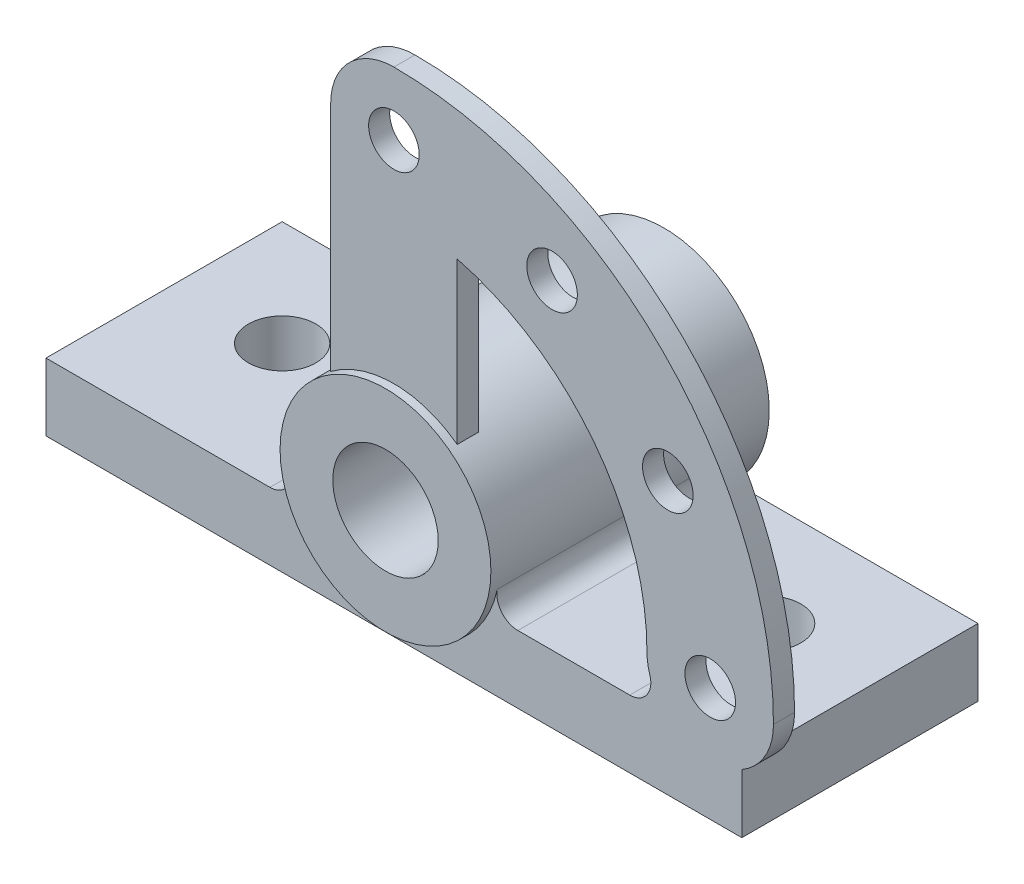
ISO-10303-21;
HEADER;
FILE_DESCRIPTION(('STEP AP214'),'2;1');
FILE_NAME('part.step','',(''),(''),'','','');
FILE_SCHEMA(('AUTOMOTIVE_DESIGN { 1 0 10303 214 1 1 1 1 }'));
ENDSEC;
DATA;
#1=APPLICATION_CONTEXT('core data for automotive mechanical design processes');
#2=APPLICATION_PROTOCOL_DEFINITION('international standard','automotive_design',2000,#1);
#3=PRODUCT_CONTEXT('',#1,'mechanical');
#4=PRODUCT('Part','Part','',(#3));
#5=PRODUCT_RELATED_PRODUCT_CATEGORY('part','',(#4));
#6=PRODUCT_DEFINITION_FORMATION('','',#4);
#7=PRODUCT_DEFINITION_CONTEXT('part definition',#1,'design');
#8=PRODUCT_DEFINITION('design','',#6,#7);
#9=PRODUCT_DEFINITION_SHAPE('','',#8);
#10=(LENGTH_UNIT() NAMED_UNIT(*) SI_UNIT(.MILLI.,.METRE.));
#11=(NAMED_UNIT(*) PLANE_ANGLE_UNIT() SI_UNIT($,.RADIAN.));
#12=(NAMED_UNIT(*) SI_UNIT($,.STERADIAN.) SOLID_ANGLE_UNIT());
#13=UNCERTAINTY_MEASURE_WITH_UNIT(LENGTH_MEASURE(1.E-05),#10,'distance_accuracy_value','');
#14=(GEOMETRIC_REPRESENTATION_CONTEXT(3) GLOBAL_UNCERTAINTY_ASSIGNED_CONTEXT((#13)) GLOBAL_UNIT_ASSIGNED_CONTEXT((#10,
#11,#12)) REPRESENTATION_CONTEXT('',''));
#15=CARTESIAN_POINT('',(0.,0.,0.));
#16=DIRECTION('',(0.,0.,1.));
#17=DIRECTION('',(1.,0.,0.));
#18=AXIS2_PLACEMENT_3D('',#15,#16,#17);
#19=CARTESIAN_POINT('',(165.,16.,56.));
#20=DIRECTION('',(0.,-1.,0.));
#21=DIRECTION('',(0.,0.,-1.));
#22=AXIS2_PLACEMENT_3D('',#19,#20,#21);
#23=PLANE('',#22);
#24=CARTESIAN_POINT('',(140.,16.,25.));
#25=DIRECTION('',(0.,1.,0.));
#26=DIRECTION('',(0.,0.,1.));
#27=AXIS2_PLACEMENT_3D('',#24,#25,#26);
#28=CIRCLE('',#27,8.00000000000001);
#29=CARTESIAN_POINT('',(140.,16.,33.));
#30=VERTEX_POINT('',#29);
#31=EDGE_CURVE('E445',#30,#30,#28,.T.);
#32=ORIENTED_EDGE('',*,*,#31,.F.);
#33=EDGE_LOOP('',(#32));
#34=FACE_BOUND('',#33,.T.);
#35=DIRECTION('',(-1.,0.,0.));
#36=VECTOR('',#35,1.);
#37=CARTESIAN_POINT('',(165.,16.,56.));
#38=LINE('',#37,#36);
#39=CARTESIAN_POINT('',(138.421215971661,16.,56.));
#40=VERTEX_POINT('',#39);
#41=CARTESIAN_POINT('',(111.893876913398,16.,56.));
#42=VERTEX_POINT('',#41);
#43=EDGE_CURVE('E291',#40,#42,#38,.T.);
#44=ORIENTED_EDGE('',*,*,#43,.F.);
#45=DIRECTION('',(0.,0.,1.));
#46=VECTOR('',#45,1.);
#47=CARTESIAN_POINT('',(138.421215971661,16.,51.));
#48=LINE('',#47,#46);
#49=CARTESIAN_POINT('',(138.421215971661,16.,51.));
#50=VERTEX_POINT('',#49);
#51=EDGE_CURVE('E333',#40,#50,#48,.F.);
#52=ORIENTED_EDGE('',*,*,#51,.T.);
#53=DIRECTION('',(-1.,0.,0.));
#54=VECTOR('',#53,1.);
#55=CARTESIAN_POINT('',(165.,16.,51.));
#56=LINE('',#55,#54);
#57=CARTESIAN_POINT('',(165.,16.,51.));
#58=VERTEX_POINT('',#57);
#59=EDGE_CURVE('E264',#58,#50,#56,.T.);
#60=ORIENTED_EDGE('',*,*,#59,.F.);
#61=DIRECTION('',(0.,0.,-1.));
#62=VECTOR('',#61,1.);
#63=CARTESIAN_POINT('',(165.,16.,56.));
#64=LINE('',#63,#62);
#65=CARTESIAN_POINT('',(165.,16.,0.));
#66=VERTEX_POINT('',#65);
#67=EDGE_CURVE('E307',#58,#66,#64,.T.);
#68=ORIENTED_EDGE('',*,*,#67,.T.);
#69=DIRECTION('',(-1.,0.,0.));
#70=VECTOR('',#69,1.);
#71=CARTESIAN_POINT('',(165.,16.,0.));
#72=LINE('',#71,#70);
#73=CARTESIAN_POINT('',(111.893876913398,16.,0.));
#74=VERTEX_POINT('',#73);
#75=EDGE_CURVE('E290',#66,#74,#72,.T.);
#76=ORIENTED_EDGE('',*,*,#75,.T.);
#77=DIRECTION('',(0.,0.,1.));
#78=VECTOR('',#77,1.);
#79=CARTESIAN_POINT('',(111.893876913398,16.,56.));
#80=LINE('',#79,#78);
#81=EDGE_CURVE('E329',#74,#42,#80,.T.);
#82=ORIENTED_EDGE('',*,*,#81,.T.);
#83=EDGE_LOOP('',(#44,#52,#60,#68,#76,#82));
#84=FACE_BOUND('',#83,.T.);
#85=ADVANCED_FACE('F43',(#34,#84),#23,.F.);
#86=CARTESIAN_POINT('',(165.,0.,56.));
#87=DIRECTION('',(-1.,0.,0.));
#88=DIRECTION('',(0.,0.,1.));
#89=AXIS2_PLACEMENT_3D('',#86,#87,#88);
#90=PLANE('',#89);
#91=DIRECTION('',(0.,0.,-1.));
#92=VECTOR('',#91,1.);
#93=CARTESIAN_POINT('',(165.,14.0096189432334,56.));
#94=LINE('',#93,#92);
#95=CARTESIAN_POINT('',(165.,14.0096189432334,56.));
#96=VERTEX_POINT('',#95);
#97=CARTESIAN_POINT('',(165.,14.0096189432334,51.));
#98=VERTEX_POINT('',#97);
#99=EDGE_CURVE('E268',#96,#98,#94,.T.);
#100=ORIENTED_EDGE('',*,*,#99,.F.);
#101=DIRECTION('',(0.,1.,0.));
#102=VECTOR('',#101,1.);
#103=CARTESIAN_POINT('',(165.,0.,56.));
#104=LINE('',#103,#102);
#105=CARTESIAN_POINT('',(165.,0.,56.));
#106=VERTEX_POINT('',#105);
#107=EDGE_CURVE('E287',#106,#96,#104,.T.);
#108=ORIENTED_EDGE('',*,*,#107,.F.);
#109=DIRECTION('',(0.,0.,-1.));
#110=VECTOR('',#109,1.);
#111=CARTESIAN_POINT('',(165.,0.,56.));
#112=LINE('',#111,#110);
#113=CARTESIAN_POINT('',(165.,0.,0.));
#114=VERTEX_POINT('',#113);
#115=EDGE_CURVE('E311',#106,#114,#112,.T.);
#116=ORIENTED_EDGE('',*,*,#115,.T.);
#117=DIRECTION('',(0.,1.,0.));
#118=VECTOR('',#117,1.);
#119=CARTESIAN_POINT('',(165.,0.,0.));
#120=LINE('',#119,#118);
#121=EDGE_CURVE('E301',#114,#66,#120,.T.);
#122=ORIENTED_EDGE('',*,*,#121,.T.);
#123=ORIENTED_EDGE('',*,*,#67,.F.);
#124=DIRECTION('',(0.,1.,0.));
#125=VECTOR('',#124,1.);
#126=CARTESIAN_POINT('',(165.,0.,51.));
#127=LINE('',#126,#125);
#128=EDGE_CURVE('E263',#98,#58,#127,.T.);
#129=ORIENTED_EDGE('',*,*,#128,.F.);
#130=EDGE_LOOP('',(#100,#108,#116,#122,#123,#129));
#131=FACE_BOUND('',#130,.T.);
#132=ADVANCED_FACE('F380',(#131),#90,.F.);
#133=CARTESIAN_POINT('',(25.,16.,25.));
#134=DIRECTION('',(0.,1.,0.));
#135=DIRECTION('',(0.,0.,1.));
#136=AXIS2_PLACEMENT_3D('',#133,#134,#135);
#137=CIRCLE('',#136,8.);
#138=CARTESIAN_POINT('',(25.,16.,33.));
#139=VERTEX_POINT('',#138);
#140=EDGE_CURVE('E401',#139,#139,#137,.T.);
#141=ORIENTED_EDGE('',*,*,#140,.F.);
#142=EDGE_LOOP('',(#141));
#143=FACE_BOUND('',#142,.T.);
#144=CARTESIAN_POINT('',(53.1061230866019,16.,56.));
#145=VERTEX_POINT('',#144);
#146=CARTESIAN_POINT('',(0.,16.,56.));
#147=VERTEX_POINT('',#146);
#148=EDGE_CURVE('E292',#145,#147,#38,.T.);
#149=ORIENTED_EDGE('',*,*,#148,.F.);
#150=DIRECTION('',(0.,0.,1.));
#151=VECTOR('',#150,1.);
#152=CARTESIAN_POINT('',(53.1061230866019,16.,0.));
#153=LINE('',#152,#151);
#154=CARTESIAN_POINT('',(53.1061230866019,16.,0.));
#155=VERTEX_POINT('',#154);
#156=EDGE_CURVE('E318',#145,#155,#153,.F.);
#157=ORIENTED_EDGE('',*,*,#156,.T.);
#158=CARTESIAN_POINT('',(0.,16.,0.));
#159=VERTEX_POINT('',#158);
#160=EDGE_CURVE('E302',#155,#159,#72,.T.);
#161=ORIENTED_EDGE('',*,*,#160,.T.);
#162=DIRECTION('',(0.,0.,-1.));
#163=VECTOR('',#162,1.);
#164=CARTESIAN_POINT('',(0.,16.,56.));
#165=LINE('',#164,#163);
#166=EDGE_CURVE('E298',#147,#159,#165,.T.);
#167=ORIENTED_EDGE('',*,*,#166,.F.);
#168=EDGE_LOOP('',(#149,#157,#161,#167));
#169=FACE_BOUND('',#168,.T.);
#170=ADVANCED_FACE('F379',(#143,#169),#23,.F.);
#171=CARTESIAN_POINT('',(0.,16.,56.));
#172=DIRECTION('',(1.,0.,0.));
#173=DIRECTION('',(0.,0.,-1.));
#174=AXIS2_PLACEMENT_3D('',#171,#172,#173);
#175=PLANE('',#174);
#176=DIRECTION('',(0.,-1.,0.));
#177=VECTOR('',#176,1.);
#178=CARTESIAN_POINT('',(0.,16.,0.));
#179=LINE('',#178,#177);
#180=CARTESIAN_POINT('',(0.,0.,0.));
#181=VERTEX_POINT('',#180);
#182=EDGE_CURVE('E285',#159,#181,#179,.T.);
#183=ORIENTED_EDGE('',*,*,#182,.T.);
#184=DIRECTION('',(0.,0.,-1.));
#185=VECTOR('',#184,1.);
#186=CARTESIAN_POINT('',(0.,0.,56.));
#187=LINE('',#186,#185);
#188=CARTESIAN_POINT('',(0.,0.,56.));
#189=VERTEX_POINT('',#188);
#190=EDGE_CURVE('E313',#189,#181,#187,.T.);
#191=ORIENTED_EDGE('',*,*,#190,.F.);
#192=DIRECTION('',(0.,-1.,0.));
#193=VECTOR('',#192,1.);
#194=CARTESIAN_POINT('',(0.,16.,56.));
#195=LINE('',#194,#193);
#196=EDGE_CURVE('E281',#147,#189,#195,.T.);
#197=ORIENTED_EDGE('',*,*,#196,.F.);
#198=ORIENTED_EDGE('',*,*,#166,.T.);
#199=EDGE_LOOP('',(#183,#191,#197,#198));
#200=FACE_BOUND('',#199,.T.);
#201=ADVANCED_FACE('F393',(#200),#175,.F.);
#202=CARTESIAN_POINT('',(75.,0.,56.));
#203=DIRECTION('',(0.,1.,0.));
#204=DIRECTION('',(0.,0.,1.));
#205=AXIS2_PLACEMENT_3D('',#202,#203,#204);
#206=PLANE('',#205);
#207=CARTESIAN_POINT('',(140.,0.,25.));
#208=DIRECTION('',(0.,1.,0.));
#209=DIRECTION('',(0.,0.,1.));
#210=AXIS2_PLACEMENT_3D('',#207,#208,#209);
#211=CIRCLE('',#210,8.00000000000001);
#212=CARTESIAN_POINT('',(140.,0.,33.));
#213=VERTEX_POINT('',#212);
#214=EDGE_CURVE('E437',#213,#213,#211,.T.);
#215=ORIENTED_EDGE('',*,*,#214,.T.);
#216=EDGE_LOOP('',(#215));
#217=FACE_BOUND('',#216,.T.);
#218=CARTESIAN_POINT('',(25.,0.,25.));
#219=DIRECTION('',(0.,1.,0.));
#220=DIRECTION('',(0.,0.,1.));
#221=AXIS2_PLACEMENT_3D('',#218,#219,#220);
#222=CIRCLE('',#221,8.);
#223=CARTESIAN_POINT('',(25.,0.,33.));
#224=VERTEX_POINT('',#223);
#225=EDGE_CURVE('E225',#224,#224,#222,.T.);
#226=ORIENTED_EDGE('',*,*,#225,.T.);
#227=EDGE_LOOP('',(#226));
#228=FACE_BOUND('',#227,.T.);
#229=DIRECTION('',(1.,0.,0.));
#230=VECTOR('',#229,1.);
#231=CARTESIAN_POINT('',(75.,0.,0.));
#232=LINE('',#231,#230);
#233=EDGE_CURVE('E299',#181,#114,#232,.T.);
#234=ORIENTED_EDGE('',*,*,#233,.T.);
#235=ORIENTED_EDGE('',*,*,#115,.F.);
#236=DIRECTION('',(1.,0.,0.));
#237=VECTOR('',#236,1.);
#238=CARTESIAN_POINT('',(0.,0.,56.));
#239=LINE('',#238,#237);
#240=EDGE_CURVE('E288',#189,#106,#239,.T.);
#241=ORIENTED_EDGE('',*,*,#240,.F.);
#242=ORIENTED_EDGE('',*,*,#190,.T.);
#243=EDGE_LOOP('',(#234,#235,#241,#242));
#244=FACE_BOUND('',#243,.T.);
#245=ADVANCED_FACE('F400',(#217,#228,#244),#206,.F.);
#246=CARTESIAN_POINT('',(0.,0.,56.));
#247=DIRECTION('',(0.,0.,1.));
#248=DIRECTION('',(1.,0.,0.));
#249=AXIS2_PLACEMENT_3D('',#246,#247,#248);
#250=PLANE('',#249);
#251=CARTESIAN_POINT('',(157.5,27.,56.));
#252=DIRECTION('',(0.,0.,1.));
#253=DIRECTION('',(1.,0.,0.));
#254=AXIS2_PLACEMENT_3D('',#251,#252,#253);
#255=CIRCLE('',#254,15.);
#256=CARTESIAN_POINT('',(142.5,27.,56.));
#257=VERTEX_POINT('',#256);
#258=CARTESIAN_POINT('',(143.190911978746,22.5,56.));
#259=VERTEX_POINT('',#258);
#260=EDGE_CURVE('E198',#257,#259,#255,.T.);
#261=ORIENTED_EDGE('',*,*,#260,.T.);
#262=CARTESIAN_POINT('',(138.421215971661,21.,56.));
#263=DIRECTION('',(0.,0.,1.));
#264=DIRECTION('',(1.,0.,0.));
#265=AXIS2_PLACEMENT_3D('',#262,#263,#264);
#266=CIRCLE('',#265,5.);
#267=EDGE_CURVE('E337',#259,#40,#266,.F.);
#268=ORIENTED_EDGE('',*,*,#267,.T.);
#269=ORIENTED_EDGE('',*,*,#43,.T.);
#270=CARTESIAN_POINT('',(111.893876913398,21.,56.));
#271=DIRECTION('',(0.,0.,1.));
#272=DIRECTION('',(1.,0.,0.));
#273=AXIS2_PLACEMENT_3D('',#270,#271,#272);
#274=CIRCLE('',#273,5.);
#275=CARTESIAN_POINT('',(106.994897427832,22.,56.));
#276=VERTEX_POINT('',#275);
#277=EDGE_CURVE('E11',#42,#276,#274,.F.);
#278=ORIENTED_EDGE('',*,*,#277,.T.);
#279=CARTESIAN_POINT('',(82.5,27.,56.));
#280=DIRECTION('',(0.,0.,1.));
#281=DIRECTION('',(1.,0.,0.));
#282=AXIS2_PLACEMENT_3D('',#279,#280,#281);
#283=CIRCLE('',#282,25.);
#284=CARTESIAN_POINT('',(58.0051025721682,22.,56.));
#285=VERTEX_POINT('',#284);
#286=EDGE_CURVE('E68',#276,#285,#283,.F.);
#287=ORIENTED_EDGE('',*,*,#286,.T.);
#288=CARTESIAN_POINT('',(53.1061230866019,21.,56.));
#289=DIRECTION('',(0.,0.,1.));
#290=DIRECTION('',(1.,0.,0.));
#291=AXIS2_PLACEMENT_3D('',#288,#289,#290);
#292=CIRCLE('',#291,5.);
#293=EDGE_CURVE('E321',#285,#145,#292,.F.);
#294=ORIENTED_EDGE('',*,*,#293,.T.);
#295=ORIENTED_EDGE('',*,*,#148,.T.);
#296=ORIENTED_EDGE('',*,*,#196,.T.);
#297=ORIENTED_EDGE('',*,*,#240,.T.);
#298=ORIENTED_EDGE('',*,*,#107,.T.);
#299=CARTESIAN_POINT('',(172.5,27.,56.));
#300=VERTEX_POINT('',#299);
#301=EDGE_CURVE('E193',#96,#300,#255,.T.);
#302=ORIENTED_EDGE('',*,*,#301,.T.);
#303=CARTESIAN_POINT('',(82.5,27.,56.));
#304=DIRECTION('',(0.,0.,1.));
#305=DIRECTION('',(1.,0.,0.));
#306=AXIS2_PLACEMENT_3D('',#303,#304,#305);
#307=CIRCLE('',#306,90.);
#308=CARTESIAN_POINT('',(82.5,117.,56.));
#309=VERTEX_POINT('',#308);
#310=EDGE_CURVE('E197',#300,#309,#307,.T.);
#311=ORIENTED_EDGE('',*,*,#310,.T.);
#312=CARTESIAN_POINT('',(82.5,102.,56.));
#313=DIRECTION('',(0.,0.,1.));
#314=DIRECTION('',(1.,0.,0.));
#315=AXIS2_PLACEMENT_3D('',#312,#313,#314);
#316=CIRCLE('',#315,15.);
#317=CARTESIAN_POINT('',(67.5,102.,56.));
#318=VERTEX_POINT('',#317);
#319=EDGE_CURVE('E205',#309,#318,#316,.T.);
#320=ORIENTED_EDGE('',*,*,#319,.T.);
#321=DIRECTION('',(0.,-1.,0.));
#322=VECTOR('',#321,1.);
#323=CARTESIAN_POINT('',(67.5,0.,56.));
#324=LINE('',#323,#322);
#325=CARTESIAN_POINT('',(67.5,47.,56.));
#326=VERTEX_POINT('',#325);
#327=EDGE_CURVE('E202',#318,#326,#324,.T.);
#328=ORIENTED_EDGE('',*,*,#327,.T.);
#329=CARTESIAN_POINT('',(82.5,27.,56.));
#330=DIRECTION('',(0.,0.,1.));
#331=DIRECTION('',(1.,0.,0.));
#332=AXIS2_PLACEMENT_3D('',#329,#330,#331);
#333=CIRCLE('',#332,25.);
#334=CARTESIAN_POINT('',(97.5,47.,56.));
#335=VERTEX_POINT('',#334);
#336=EDGE_CURVE('E188',#335,#326,#333,.T.);
#337=ORIENTED_EDGE('',*,*,#336,.F.);
#338=DIRECTION('',(0.,-1.,0.));
#339=VECTOR('',#338,1.);
#340=CARTESIAN_POINT('',(97.5,0.,56.));
#341=LINE('',#340,#339);
#342=CARTESIAN_POINT('',(97.5,85.0947501931113,56.));
#343=VERTEX_POINT('',#342);
#344=EDGE_CURVE('E175',#343,#335,#341,.T.);
#345=ORIENTED_EDGE('',*,*,#344,.F.);
#346=CARTESIAN_POINT('',(82.5,27.,56.));
#347=DIRECTION('',(0.,0.,1.));
#348=DIRECTION('',(1.,0.,0.));
#349=AXIS2_PLACEMENT_3D('',#346,#347,#348);
#350=CIRCLE('',#349,60.);
#351=EDGE_CURVE('E189',#257,#343,#350,.T.);
#352=ORIENTED_EDGE('',*,*,#351,.F.);
#353=EDGE_LOOP('',(#261,#268,#269,#278,#287,#294,#295,#296,#297,#298,#302,#311,#320,#328,#337,
#345,#352));
#354=FACE_BOUND('',#353,.T.);
#355=CARTESIAN_POINT('',(82.5,102.,56.));
#356=DIRECTION('',(0.,0.,1.));
#357=DIRECTION('',(1.,0.,0.));
#358=AXIS2_PLACEMENT_3D('',#355,#356,#357);
#359=CIRCLE('',#358,6.);
#360=CARTESIAN_POINT('',(88.5,102.,56.));
#361=VERTEX_POINT('',#360);
#362=EDGE_CURVE('E212',#361,#361,#359,.T.);
#363=ORIENTED_EDGE('',*,*,#362,.F.);
#364=EDGE_LOOP('',(#363));
#365=FACE_BOUND('',#364,.T.);
#366=CARTESIAN_POINT('',(157.5,27.,56.));
#367=DIRECTION('',(0.,0.,1.));
#368=DIRECTION('',(1.,0.,0.));
#369=AXIS2_PLACEMENT_3D('',#366,#367,#368);
#370=CIRCLE('',#369,5.99999999999999);
#371=CARTESIAN_POINT('',(163.5,27.,56.));
#372=VERTEX_POINT('',#371);
#373=EDGE_CURVE('E211',#372,#372,#370,.T.);
#374=ORIENTED_EDGE('',*,*,#373,.F.);
#375=EDGE_LOOP('',(#374));
#376=FACE_BOUND('',#375,.T.);
#377=CARTESIAN_POINT('',(147.451905283833,64.5000000000001,56.));
#378=DIRECTION('',(0.,0.,1.));
#379=DIRECTION('',(1.,0.,0.));
#380=AXIS2_PLACEMENT_3D('',#377,#378,#379);
#381=CIRCLE('',#380,6.00000000000002);
#382=CARTESIAN_POINT('',(153.451905283833,64.5000000000001,56.));
#383=VERTEX_POINT('',#382);
#384=EDGE_CURVE('E209',#383,#383,#381,.T.);
#385=ORIENTED_EDGE('',*,*,#384,.F.);
#386=EDGE_LOOP('',(#385));
#387=FACE_BOUND('',#386,.T.);
#388=CARTESIAN_POINT('',(120.,91.951905283833,56.));
#389=DIRECTION('',(0.,0.,1.));
#390=DIRECTION('',(1.,0.,0.));
#391=AXIS2_PLACEMENT_3D('',#388,#389,#390);
#392=CIRCLE('',#391,5.99999999999999);
#393=CARTESIAN_POINT('',(126.,91.951905283833,56.));
#394=VERTEX_POINT('',#393);
#395=EDGE_CURVE('E207',#394,#394,#392,.T.);
#396=ORIENTED_EDGE('',*,*,#395,.F.);
#397=EDGE_LOOP('',(#396));
#398=FACE_BOUND('',#397,.T.);
#399=ADVANCED_FACE('F187',(#354,#365,#376,#387,#398),#250,.T.);
#400=CARTESIAN_POINT('',(0.,0.,0.));
#401=DIRECTION('',(0.,0.,1.));
#402=DIRECTION('',(1.,0.,0.));
#403=AXIS2_PLACEMENT_3D('',#400,#401,#402);
#404=PLANE('',#403);
#405=CARTESIAN_POINT('',(82.5,27.,0.));
#406=DIRECTION('',(0.,0.,1.));
#407=DIRECTION('',(1.,0.,0.));
#408=AXIS2_PLACEMENT_3D('',#405,#406,#407);
#409=CIRCLE('',#408,25.);
#410=CARTESIAN_POINT('',(106.994897427832,22.,0.));
#411=VERTEX_POINT('',#410);
#412=CARTESIAN_POINT('',(58.0051025721682,22.,0.));
#413=VERTEX_POINT('',#412);
#414=EDGE_CURVE('E59',#411,#413,#409,.F.);
#415=ORIENTED_EDGE('',*,*,#414,.F.);
#416=CARTESIAN_POINT('',(111.893876913398,21.,0.));
#417=DIRECTION('',(0.,0.,1.));
#418=DIRECTION('',(1.,0.,0.));
#419=AXIS2_PLACEMENT_3D('',#416,#417,#418);
#420=CIRCLE('',#419,5.);
#421=EDGE_CURVE('E51',#411,#74,#420,.T.);
#422=ORIENTED_EDGE('',*,*,#421,.T.);
#423=ORIENTED_EDGE('',*,*,#75,.F.);
#424=ORIENTED_EDGE('',*,*,#121,.F.);
#425=ORIENTED_EDGE('',*,*,#233,.F.);
#426=ORIENTED_EDGE('',*,*,#182,.F.);
#427=ORIENTED_EDGE('',*,*,#160,.F.);
#428=CARTESIAN_POINT('',(53.1061230866019,21.,0.));
#429=DIRECTION('',(0.,0.,1.));
#430=DIRECTION('',(1.,0.,0.));
#431=AXIS2_PLACEMENT_3D('',#428,#429,#430);
#432=CIRCLE('',#431,5.);
#433=EDGE_CURVE('E323',#155,#413,#432,.T.);
#434=ORIENTED_EDGE('',*,*,#433,.T.);
#435=EDGE_LOOP('',(#415,#422,#423,#424,#425,#426,#427,#434));
#436=FACE_BOUND('',#435,.T.);
#437=ADVANCED_FACE('F338',(#436),#404,.F.);
#438=CARTESIAN_POINT('',(82.5,27.,58.));
#439=DIRECTION('',(0.,0.,1.));
#440=DIRECTION('',(1.,0.,0.));
#441=AXIS2_PLACEMENT_3D('',#438,#439,#440);
#442=PLANE('',#441);
#443=CARTESIAN_POINT('',(82.5,27.,58.));
#444=DIRECTION('',(0.,0.,1.));
#445=DIRECTION('',(1.,0.,0.));
#446=AXIS2_PLACEMENT_3D('',#443,#444,#445);
#447=CIRCLE('',#446,25.);
#448=CARTESIAN_POINT('',(107.5,27.,58.));
#449=VERTEX_POINT('',#448);
#450=EDGE_CURVE('E279',#449,#449,#447,.T.);
#451=ORIENTED_EDGE('',*,*,#450,.T.);
#452=EDGE_LOOP('',(#451));
#453=FACE_BOUND('',#452,.T.);
#454=CARTESIAN_POINT('',(82.5,27.,58.));
#455=DIRECTION('',(0.,0.,1.));
#456=DIRECTION('',(1.,0.,0.));
#457=AXIS2_PLACEMENT_3D('',#454,#455,#456);
#458=CIRCLE('',#457,12.5);
#459=CARTESIAN_POINT('',(95.,27.,58.));
#460=VERTEX_POINT('',#459);
#461=EDGE_CURVE('E269',#460,#460,#458,.T.);
#462=ORIENTED_EDGE('',*,*,#461,.F.);
#463=EDGE_LOOP('',(#462));
#464=FACE_BOUND('',#463,.T.);
#465=ADVANCED_FACE('F495',(#453,#464),#442,.T.);
#466=CARTESIAN_POINT('',(82.5,27.,-8.));
#467=DIRECTION('',(0.,0.,1.));
#468=DIRECTION('',(1.,0.,0.));
#469=AXIS2_PLACEMENT_3D('',#466,#467,#468);
#470=PLANE('',#469);
#471=CARTESIAN_POINT('',(82.5,27.,-8.));
#472=DIRECTION('',(0.,0.,1.));
#473=DIRECTION('',(1.,0.,0.));
#474=AXIS2_PLACEMENT_3D('',#471,#472,#473);
#475=CIRCLE('',#474,25.);
#476=CARTESIAN_POINT('',(107.5,27.,-8.));
#477=VERTEX_POINT('',#476);
#478=EDGE_CURVE('E271',#477,#477,#475,.T.);
#479=ORIENTED_EDGE('',*,*,#478,.F.);
#480=EDGE_LOOP('',(#479));
#481=FACE_BOUND('',#480,.T.);
#482=CARTESIAN_POINT('',(82.5,27.,-8.));
#483=DIRECTION('',(0.,0.,1.));
#484=DIRECTION('',(1.,0.,0.));
#485=AXIS2_PLACEMENT_3D('',#482,#483,#484);
#486=CIRCLE('',#485,12.5);
#487=CARTESIAN_POINT('',(95.,27.,-8.));
#488=VERTEX_POINT('',#487);
#489=EDGE_CURVE('E267',#488,#488,#486,.T.);
#490=ORIENTED_EDGE('',*,*,#489,.T.);
#491=EDGE_LOOP('',(#490));
#492=FACE_BOUND('',#491,.T.);
#493=ADVANCED_FACE('F492',(#481,#492),#470,.F.);
#494=CARTESIAN_POINT('',(82.5,27.,58.));
#495=DIRECTION('',(0.,0.,-1.));
#496=DIRECTION('',(-1.,0.,0.));
#497=AXIS2_PLACEMENT_3D('',#494,#495,#496);
#498=CYLINDRICAL_SURFACE('',#497,25.);
#499=DIRECTION('',(0.,0.,-1.));
#500=VECTOR('',#499,1.);
#501=CARTESIAN_POINT('',(97.5,47.,56.));
#502=LINE('',#501,#500);
#503=CARTESIAN_POINT('',(97.5,47.,51.));
#504=VERTEX_POINT('',#503);
#505=EDGE_CURVE('E177',#335,#504,#502,.T.);
#506=ORIENTED_EDGE('',*,*,#505,.F.);
#507=ORIENTED_EDGE('',*,*,#336,.T.);
#508=DIRECTION('',(0.,0.,-1.));
#509=VECTOR('',#508,1.);
#510=CARTESIAN_POINT('',(67.5,47.,56.));
#511=LINE('',#510,#509);
#512=CARTESIAN_POINT('',(67.5,47.,51.));
#513=VERTEX_POINT('',#512);
#514=EDGE_CURVE('E216',#326,#513,#511,.T.);
#515=ORIENTED_EDGE('',*,*,#514,.T.);
#516=CARTESIAN_POINT('',(82.5,27.,51.));
#517=DIRECTION('',(0.,0.,1.));
#518=DIRECTION('',(1.,0.,0.));
#519=AXIS2_PLACEMENT_3D('',#516,#517,#518);
#520=CIRCLE('',#519,25.);
#521=EDGE_CURVE('E219',#504,#513,#520,.T.);
#522=ORIENTED_EDGE('',*,*,#521,.F.);
#523=EDGE_LOOP('',(#506,#507,#515,#522));
#524=FACE_BOUND('',#523,.T.);
#525=DIRECTION('',(0.,0.,-1.));
#526=VECTOR('',#525,1.);
#527=CARTESIAN_POINT('',(106.994897427832,22.,58.));
#528=LINE('',#527,#526);
#529=EDGE_CURVE('E332',#276,#411,#528,.T.);
#530=ORIENTED_EDGE('',*,*,#529,.T.);
#531=ORIENTED_EDGE('',*,*,#414,.T.);
#532=DIRECTION('',(0.,0.,-1.));
#533=VECTOR('',#532,1.);
#534=CARTESIAN_POINT('',(58.0051025721682,22.,58.));
#535=LINE('',#534,#533);
#536=EDGE_CURVE('E319',#413,#285,#535,.F.);
#537=ORIENTED_EDGE('',*,*,#536,.T.);
#538=ORIENTED_EDGE('',*,*,#286,.F.);
#539=EDGE_LOOP('',(#530,#531,#537,#538));
#540=FACE_BOUND('',#539,.T.);
#541=ORIENTED_EDGE('',*,*,#450,.F.);
#542=EDGE_LOOP('',(#541));
#543=FACE_BOUND('',#542,.T.);
#544=ORIENTED_EDGE('',*,*,#478,.T.);
#545=EDGE_LOOP('',(#544));
#546=FACE_BOUND('',#545,.T.);
#547=ADVANCED_FACE('F371',(#524,#540,#543,#546),#498,.T.);
#548=CARTESIAN_POINT('',(82.5,27.,58.));
#549=DIRECTION('',(0.,0.,-1.));
#550=DIRECTION('',(-1.,0.,0.));
#551=AXIS2_PLACEMENT_3D('',#548,#549,#550);
#552=CYLINDRICAL_SURFACE('',#551,12.5);
#553=ORIENTED_EDGE('',*,*,#461,.T.);
#554=EDGE_LOOP('',(#553));
#555=FACE_BOUND('',#554,.T.);
#556=ORIENTED_EDGE('',*,*,#489,.F.);
#557=EDGE_LOOP('',(#556));
#558=FACE_BOUND('',#557,.T.);
#559=ADVANCED_FACE('F365',(#555,#558),#552,.F.);
#560=CARTESIAN_POINT('',(157.5,27.,56.));
#561=DIRECTION('',(0.,0.,-1.));
#562=DIRECTION('',(-1.,0.,0.));
#563=AXIS2_PLACEMENT_3D('',#560,#561,#562);
#564=CYLINDRICAL_SURFACE('',#563,15.);
#565=CARTESIAN_POINT('',(157.5,27.,51.));
#566=DIRECTION('',(0.,0.,1.));
#567=DIRECTION('',(1.,0.,0.));
#568=AXIS2_PLACEMENT_3D('',#565,#566,#567);
#569=CIRCLE('',#568,15.);
#570=CARTESIAN_POINT('',(142.5,27.,51.));
#571=VERTEX_POINT('',#570);
#572=CARTESIAN_POINT('',(143.190911978746,22.5,51.));
#573=VERTEX_POINT('',#572);
#574=EDGE_CURVE('E227',#571,#573,#569,.T.);
#575=ORIENTED_EDGE('',*,*,#574,.T.);
#576=DIRECTION('',(0.,0.,-1.));
#577=VECTOR('',#576,1.);
#578=CARTESIAN_POINT('',(143.190911978746,22.5,56.));
#579=LINE('',#578,#577);
#580=EDGE_CURVE('E328',#573,#259,#579,.F.);
#581=ORIENTED_EDGE('',*,*,#580,.T.);
#582=ORIENTED_EDGE('',*,*,#260,.F.);
#583=DIRECTION('',(0.,0.,-1.));
#584=VECTOR('',#583,1.);
#585=CARTESIAN_POINT('',(142.5,27.,56.));
#586=LINE('',#585,#584);
#587=EDGE_CURVE('E179',#257,#571,#586,.T.);
#588=ORIENTED_EDGE('',*,*,#587,.T.);
#589=EDGE_LOOP('',(#575,#581,#582,#588));
#590=FACE_BOUND('',#589,.T.);
#591=ADVANCED_FACE('F360',(#590),#564,.T.);
#592=ORIENTED_EDGE('',*,*,#301,.F.);
#593=ORIENTED_EDGE('',*,*,#99,.T.);
#594=CARTESIAN_POINT('',(172.5,27.,51.));
#595=VERTEX_POINT('',#594);
#596=EDGE_CURVE('E228',#98,#595,#569,.T.);
#597=ORIENTED_EDGE('',*,*,#596,.T.);
#598=DIRECTION('',(0.,0.,-1.));
#599=VECTOR('',#598,1.);
#600=CARTESIAN_POINT('',(172.5,27.,56.));
#601=LINE('',#600,#599);
#602=EDGE_CURVE('E259',#300,#595,#601,.T.);
#603=ORIENTED_EDGE('',*,*,#602,.F.);
#604=EDGE_LOOP('',(#592,#593,#597,#603));
#605=FACE_BOUND('',#604,.T.);
#606=ADVANCED_FACE('F363',(#605),#564,.T.);
#607=CARTESIAN_POINT('',(0.,0.,51.));
#608=DIRECTION('',(0.,0.,1.));
#609=DIRECTION('',(1.,0.,0.));
#610=AXIS2_PLACEMENT_3D('',#607,#608,#609);
#611=PLANE('',#610);
#612=CARTESIAN_POINT('',(120.,91.951905283833,51.));
#613=DIRECTION('',(0.,0.,1.));
#614=DIRECTION('',(1.,0.,0.));
#615=AXIS2_PLACEMENT_3D('',#612,#613,#614);
#616=CIRCLE('',#615,5.99999999999999);
#617=CARTESIAN_POINT('',(126.,91.951905283833,51.));
#618=VERTEX_POINT('',#617);
#619=EDGE_CURVE('E240',#618,#618,#616,.T.);
#620=ORIENTED_EDGE('',*,*,#619,.T.);
#621=EDGE_LOOP('',(#620));
#622=FACE_BOUND('',#621,.T.);
#623=CARTESIAN_POINT('',(147.451905283833,64.5000000000001,51.));
#624=DIRECTION('',(0.,0.,1.));
#625=DIRECTION('',(1.,0.,0.));
#626=AXIS2_PLACEMENT_3D('',#623,#624,#625);
#627=CIRCLE('',#626,6.00000000000002);
#628=CARTESIAN_POINT('',(153.451905283833,64.5000000000001,51.));
#629=VERTEX_POINT('',#628);
#630=EDGE_CURVE('E239',#629,#629,#627,.T.);
#631=ORIENTED_EDGE('',*,*,#630,.T.);
#632=EDGE_LOOP('',(#631));
#633=FACE_BOUND('',#632,.T.);
#634=CARTESIAN_POINT('',(157.5,27.,51.));
#635=DIRECTION('',(0.,0.,1.));
#636=DIRECTION('',(1.,0.,0.));
#637=AXIS2_PLACEMENT_3D('',#634,#635,#636);
#638=CIRCLE('',#637,5.99999999999999);
#639=CARTESIAN_POINT('',(163.5,27.,51.));
#640=VERTEX_POINT('',#639);
#641=EDGE_CURVE('E243',#640,#640,#638,.T.);
#642=ORIENTED_EDGE('',*,*,#641,.T.);
#643=EDGE_LOOP('',(#642));
#644=FACE_BOUND('',#643,.T.);
#645=CARTESIAN_POINT('',(82.5,102.,51.));
#646=DIRECTION('',(0.,0.,1.));
#647=DIRECTION('',(1.,0.,0.));
#648=AXIS2_PLACEMENT_3D('',#645,#646,#647);
#649=CIRCLE('',#648,6.);
#650=CARTESIAN_POINT('',(88.5,102.,51.));
#651=VERTEX_POINT('',#650);
#652=EDGE_CURVE('E246',#651,#651,#649,.T.);
#653=ORIENTED_EDGE('',*,*,#652,.T.);
#654=EDGE_LOOP('',(#653));
#655=FACE_BOUND('',#654,.T.);
#656=ORIENTED_EDGE('',*,*,#128,.T.);
#657=ORIENTED_EDGE('',*,*,#59,.T.);
#658=CARTESIAN_POINT('',(138.421215971661,21.,51.));
#659=DIRECTION('',(0.,0.,1.));
#660=DIRECTION('',(1.,0.,0.));
#661=AXIS2_PLACEMENT_3D('',#658,#659,#660);
#662=CIRCLE('',#661,5.);
#663=EDGE_CURVE('E336',#50,#573,#662,.T.);
#664=ORIENTED_EDGE('',*,*,#663,.T.);
#665=ORIENTED_EDGE('',*,*,#574,.F.);
#666=CARTESIAN_POINT('',(82.5,27.,51.));
#667=DIRECTION('',(0.,0.,1.));
#668=DIRECTION('',(1.,0.,0.));
#669=AXIS2_PLACEMENT_3D('',#666,#667,#668);
#670=CIRCLE('',#669,60.);
#671=CARTESIAN_POINT('',(97.5,85.0947501931113,51.));
#672=VERTEX_POINT('',#671);
#673=EDGE_CURVE('E222',#571,#672,#670,.T.);
#674=ORIENTED_EDGE('',*,*,#673,.T.);
#675=DIRECTION('',(0.,-1.,0.));
#676=VECTOR('',#675,1.);
#677=CARTESIAN_POINT('',(97.5,0.,51.));
#678=LINE('',#677,#676);
#679=EDGE_CURVE('E172',#672,#504,#678,.T.);
#680=ORIENTED_EDGE('',*,*,#679,.T.);
#681=ORIENTED_EDGE('',*,*,#521,.T.);
#682=DIRECTION('',(0.,-1.,0.));
#683=VECTOR('',#682,1.);
#684=CARTESIAN_POINT('',(67.5,0.,51.));
#685=LINE('',#684,#683);
#686=CARTESIAN_POINT('',(67.5,102.,51.));
#687=VERTEX_POINT('',#686);
#688=EDGE_CURVE('E234',#687,#513,#685,.T.);
#689=ORIENTED_EDGE('',*,*,#688,.F.);
#690=CARTESIAN_POINT('',(82.5,102.,51.));
#691=DIRECTION('',(0.,0.,1.));
#692=DIRECTION('',(1.,0.,0.));
#693=AXIS2_PLACEMENT_3D('',#690,#691,#692);
#694=CIRCLE('',#693,15.);
#695=CARTESIAN_POINT('',(82.5,117.,51.));
#696=VERTEX_POINT('',#695);
#697=EDGE_CURVE('E235',#696,#687,#694,.T.);
#698=ORIENTED_EDGE('',*,*,#697,.F.);
#699=CARTESIAN_POINT('',(82.5,27.,51.));
#700=DIRECTION('',(0.,0.,1.));
#701=DIRECTION('',(1.,0.,0.));
#702=AXIS2_PLACEMENT_3D('',#699,#700,#701);
#703=CIRCLE('',#702,90.);
#704=EDGE_CURVE('E229',#595,#696,#703,.T.);
#705=ORIENTED_EDGE('',*,*,#704,.F.);
#706=ORIENTED_EDGE('',*,*,#596,.F.);
#707=EDGE_LOOP('',(#656,#657,#664,#665,#674,#680,#681,#689,#698,#705,#706));
#708=FACE_BOUND('',#707,.T.);
#709=ADVANCED_FACE('F357',(#622,#633,#644,#655,#708),#611,.F.);
#710=CARTESIAN_POINT('',(97.5,0.,56.));
#711=DIRECTION('',(1.,0.,0.));
#712=DIRECTION('',(0.,0.,-1.));
#713=AXIS2_PLACEMENT_3D('',#710,#711,#712);
#714=PLANE('',#713);
#715=ORIENTED_EDGE('',*,*,#679,.F.);
#716=DIRECTION('',(0.,0.,-1.));
#717=VECTOR('',#716,1.);
#718=CARTESIAN_POINT('',(97.5,85.0947501931113,56.));
#719=LINE('',#718,#717);
#720=EDGE_CURVE('E166',#343,#672,#719,.T.);
#721=ORIENTED_EDGE('',*,*,#720,.F.);
#722=ORIENTED_EDGE('',*,*,#344,.T.);
#723=ORIENTED_EDGE('',*,*,#505,.T.);
#724=EDGE_LOOP('',(#715,#721,#722,#723));
#725=FACE_BOUND('',#724,.T.);
#726=ADVANCED_FACE('F167',(#725),#714,.T.);
#727=CARTESIAN_POINT('',(82.5,27.,56.));
#728=DIRECTION('',(0.,0.,-1.));
#729=DIRECTION('',(-1.,0.,0.));
#730=AXIS2_PLACEMENT_3D('',#727,#728,#729);
#731=CYLINDRICAL_SURFACE('',#730,60.);
#732=ORIENTED_EDGE('',*,*,#673,.F.);
#733=ORIENTED_EDGE('',*,*,#587,.F.);
#734=ORIENTED_EDGE('',*,*,#351,.T.);
#735=ORIENTED_EDGE('',*,*,#720,.T.);
#736=EDGE_LOOP('',(#732,#733,#734,#735));
#737=FACE_BOUND('',#736,.T.);
#738=ADVANCED_FACE('F191',(#737),#731,.F.);
#739=CARTESIAN_POINT('',(82.5,27.,56.));
#740=DIRECTION('',(0.,0.,-1.));
#741=DIRECTION('',(-1.,0.,0.));
#742=AXIS2_PLACEMENT_3D('',#739,#740,#741);
#743=CYLINDRICAL_SURFACE('',#742,90.);
#744=ORIENTED_EDGE('',*,*,#704,.T.);
#745=DIRECTION('',(0.,0.,-1.));
#746=VECTOR('',#745,1.);
#747=CARTESIAN_POINT('',(82.5,117.,56.));
#748=LINE('',#747,#746);
#749=EDGE_CURVE('E254',#309,#696,#748,.T.);
#750=ORIENTED_EDGE('',*,*,#749,.F.);
#751=ORIENTED_EDGE('',*,*,#310,.F.);
#752=ORIENTED_EDGE('',*,*,#602,.T.);
#753=EDGE_LOOP('',(#744,#750,#751,#752));
#754=FACE_BOUND('',#753,.T.);
#755=ADVANCED_FACE('F428',(#754),#743,.T.);
#756=CARTESIAN_POINT('',(82.5,102.,56.));
#757=DIRECTION('',(0.,0.,-1.));
#758=DIRECTION('',(-1.,0.,0.));
#759=AXIS2_PLACEMENT_3D('',#756,#757,#758);
#760=CYLINDRICAL_SURFACE('',#759,15.);
#761=ORIENTED_EDGE('',*,*,#697,.T.);
#762=DIRECTION('',(0.,0.,-1.));
#763=VECTOR('',#762,1.);
#764=CARTESIAN_POINT('',(67.5,102.,56.));
#765=LINE('',#764,#763);
#766=EDGE_CURVE('E249',#318,#687,#765,.T.);
#767=ORIENTED_EDGE('',*,*,#766,.F.);
#768=ORIENTED_EDGE('',*,*,#319,.F.);
#769=ORIENTED_EDGE('',*,*,#749,.T.);
#770=EDGE_LOOP('',(#761,#767,#768,#769));
#771=FACE_BOUND('',#770,.T.);
#772=ADVANCED_FACE('F427',(#771),#760,.T.);
#773=CARTESIAN_POINT('',(157.5,27.,56.));
#774=DIRECTION('',(0.,0.,-1.));
#775=DIRECTION('',(-1.,0.,0.));
#776=AXIS2_PLACEMENT_3D('',#773,#774,#775);
#777=CYLINDRICAL_SURFACE('',#776,5.99999999999999);
#778=ORIENTED_EDGE('',*,*,#373,.T.);
#779=EDGE_LOOP('',(#778));
#780=FACE_BOUND('',#779,.T.);
#781=ORIENTED_EDGE('',*,*,#641,.F.);
#782=EDGE_LOOP('',(#781));
#783=FACE_BOUND('',#782,.T.);
#784=ADVANCED_FACE('F466',(#780,#783),#777,.F.);
#785=CARTESIAN_POINT('',(147.451905283833,64.5000000000001,56.));
#786=DIRECTION('',(0.,0.,-1.));
#787=DIRECTION('',(-1.,0.,0.));
#788=AXIS2_PLACEMENT_3D('',#785,#786,#787);
#789=CYLINDRICAL_SURFACE('',#788,6.00000000000002);
#790=ORIENTED_EDGE('',*,*,#384,.T.);
#791=EDGE_LOOP('',(#790));
#792=FACE_BOUND('',#791,.T.);
#793=ORIENTED_EDGE('',*,*,#630,.F.);
#794=EDGE_LOOP('',(#793));
#795=FACE_BOUND('',#794,.T.);
#796=ADVANCED_FACE('F474',(#792,#795),#789,.F.);
#797=CARTESIAN_POINT('',(120.,91.951905283833,56.));
#798=DIRECTION('',(0.,0.,-1.));
#799=DIRECTION('',(-1.,0.,0.));
#800=AXIS2_PLACEMENT_3D('',#797,#798,#799);
#801=CYLINDRICAL_SURFACE('',#800,5.99999999999999);
#802=ORIENTED_EDGE('',*,*,#395,.T.);
#803=EDGE_LOOP('',(#802));
#804=FACE_BOUND('',#803,.T.);
#805=ORIENTED_EDGE('',*,*,#619,.F.);
#806=EDGE_LOOP('',(#805));
#807=FACE_BOUND('',#806,.T.);
#808=ADVANCED_FACE('F472',(#804,#807),#801,.F.);
#809=CARTESIAN_POINT('',(67.5,0.,56.));
#810=DIRECTION('',(1.,0.,0.));
#811=DIRECTION('',(0.,0.,-1.));
#812=AXIS2_PLACEMENT_3D('',#809,#810,#811);
#813=PLANE('',#812);
#814=ORIENTED_EDGE('',*,*,#688,.T.);
#815=ORIENTED_EDGE('',*,*,#514,.F.);
#816=ORIENTED_EDGE('',*,*,#327,.F.);
#817=ORIENTED_EDGE('',*,*,#766,.T.);
#818=EDGE_LOOP('',(#814,#815,#816,#817));
#819=FACE_BOUND('',#818,.T.);
#820=ADVANCED_FACE('F434',(#819),#813,.F.);
#821=CARTESIAN_POINT('',(82.5,102.,56.));
#822=DIRECTION('',(0.,0.,-1.));
#823=DIRECTION('',(-1.,0.,0.));
#824=AXIS2_PLACEMENT_3D('',#821,#822,#823);
#825=CYLINDRICAL_SURFACE('',#824,6.);
#826=ORIENTED_EDGE('',*,*,#362,.T.);
#827=EDGE_LOOP('',(#826));
#828=FACE_BOUND('',#827,.T.);
#829=ORIENTED_EDGE('',*,*,#652,.F.);
#830=EDGE_LOOP('',(#829));
#831=FACE_BOUND('',#830,.T.);
#832=ADVANCED_FACE('F459',(#828,#831),#825,.F.);
#833=CARTESIAN_POINT('',(25.,0.,25.));
#834=DIRECTION('',(0.,1.,0.));
#835=DIRECTION('',(0.,0.,1.));
#836=AXIS2_PLACEMENT_3D('',#833,#834,#835);
#837=CYLINDRICAL_SURFACE('',#836,8.);
#838=ORIENTED_EDGE('',*,*,#225,.F.);
#839=EDGE_LOOP('',(#838));
#840=FACE_BOUND('',#839,.T.);
#841=ORIENTED_EDGE('',*,*,#140,.T.);
#842=EDGE_LOOP('',(#841));
#843=FACE_BOUND('',#842,.T.);
#844=ADVANCED_FACE('F451',(#840,#843),#837,.F.);
#845=CARTESIAN_POINT('',(140.,0.,25.));
#846=DIRECTION('',(0.,1.,0.));
#847=DIRECTION('',(0.,0.,1.));
#848=AXIS2_PLACEMENT_3D('',#845,#846,#847);
#849=CYLINDRICAL_SURFACE('',#848,8.00000000000001);
#850=ORIENTED_EDGE('',*,*,#214,.F.);
#851=EDGE_LOOP('',(#850));
#852=FACE_BOUND('',#851,.T.);
#853=ORIENTED_EDGE('',*,*,#31,.T.);
#854=EDGE_LOOP('',(#853));
#855=FACE_BOUND('',#854,.T.);
#856=ADVANCED_FACE('F448',(#852,#855),#849,.F.);
#857=CARTESIAN_POINT('',(53.1061230866019,21.,58.));
#858=DIRECTION('',(0.,0.,-1.));
#859=DIRECTION('',(-1.,0.,0.));
#860=AXIS2_PLACEMENT_3D('',#857,#858,#859);
#861=CYLINDRICAL_SURFACE('',#860,5.);
#862=ORIENTED_EDGE('',*,*,#433,.F.);
#863=ORIENTED_EDGE('',*,*,#156,.F.);
#864=ORIENTED_EDGE('',*,*,#293,.F.);
#865=ORIENTED_EDGE('',*,*,#536,.F.);
#866=EDGE_LOOP('',(#862,#863,#864,#865));
#867=FACE_BOUND('',#866,.T.);
#868=ADVANCED_FACE('F413',(#867),#861,.F.);
#869=CARTESIAN_POINT('',(138.421215971661,21.,56.));
#870=DIRECTION('',(0.,0.,-1.));
#871=DIRECTION('',(-1.,0.,0.));
#872=AXIS2_PLACEMENT_3D('',#869,#870,#871);
#873=CYLINDRICAL_SURFACE('',#872,5.);
#874=ORIENTED_EDGE('',*,*,#663,.F.);
#875=ORIENTED_EDGE('',*,*,#51,.F.);
#876=ORIENTED_EDGE('',*,*,#267,.F.);
#877=ORIENTED_EDGE('',*,*,#580,.F.);
#878=EDGE_LOOP('',(#874,#875,#876,#877));
#879=FACE_BOUND('',#878,.T.);
#880=ADVANCED_FACE('F351',(#879),#873,.F.);
#881=CARTESIAN_POINT('',(111.893876913398,21.,58.));
#882=DIRECTION('',(0.,0.,-1.));
#883=DIRECTION('',(-1.,0.,0.));
#884=AXIS2_PLACEMENT_3D('',#881,#882,#883);
#885=CYLINDRICAL_SURFACE('',#884,5.);
#886=ORIENTED_EDGE('',*,*,#277,.F.);
#887=ORIENTED_EDGE('',*,*,#81,.F.);
#888=ORIENTED_EDGE('',*,*,#421,.F.);
#889=ORIENTED_EDGE('',*,*,#529,.F.);
#890=EDGE_LOOP('',(#886,#887,#888,#889));
#891=FACE_BOUND('',#890,.T.);
#892=ADVANCED_FACE('F44',(#891),#885,.F.);
#893=CLOSED_SHELL('',(#85,#132,#170,#201,#245,#399,#437,#465,#493,#547,#559,#591,#606,#709,#726,
#738,#755,#772,#784,#796,#808,#820,#832,#844,#856,#868,#880,#892));
#894=MANIFOLD_SOLID_BREP('B2',#893);
#895=ADVANCED_BREP_SHAPE_REPRESENTATION('',(#18,#894),#14);
#896=SHAPE_DEFINITION_REPRESENTATION(#9,#895);
ENDSEC;
END-ISO-10303-21;
